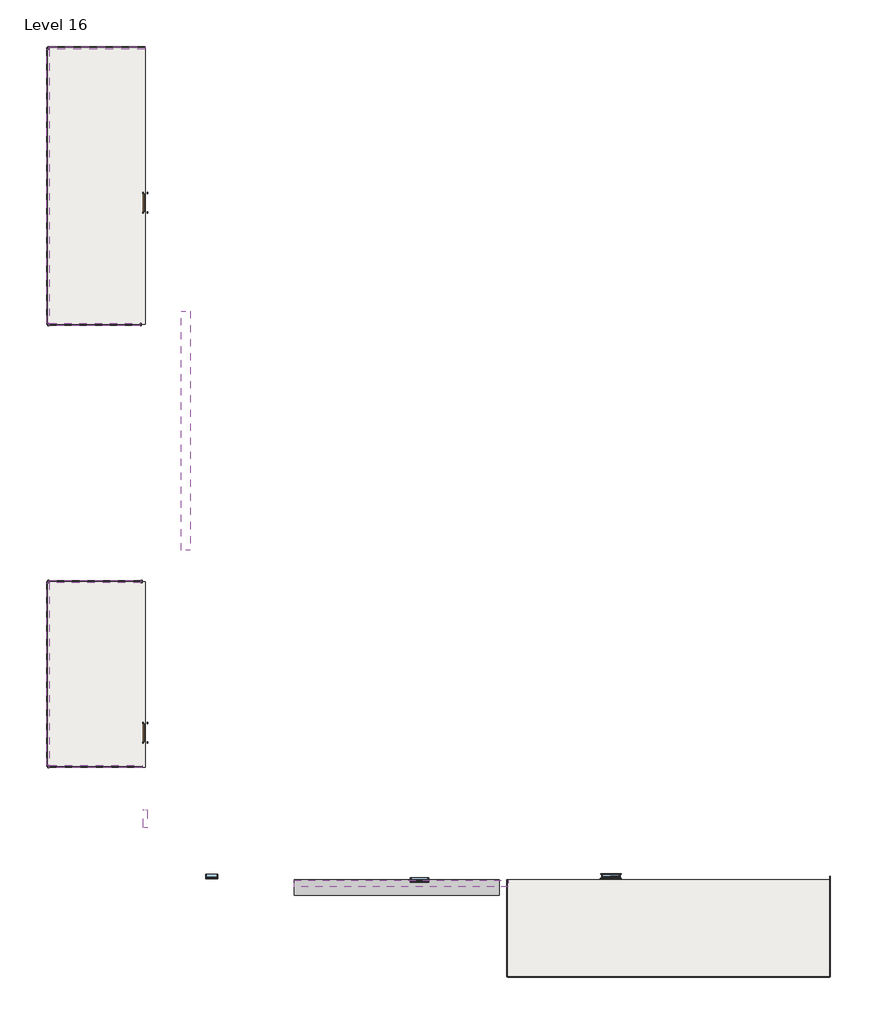
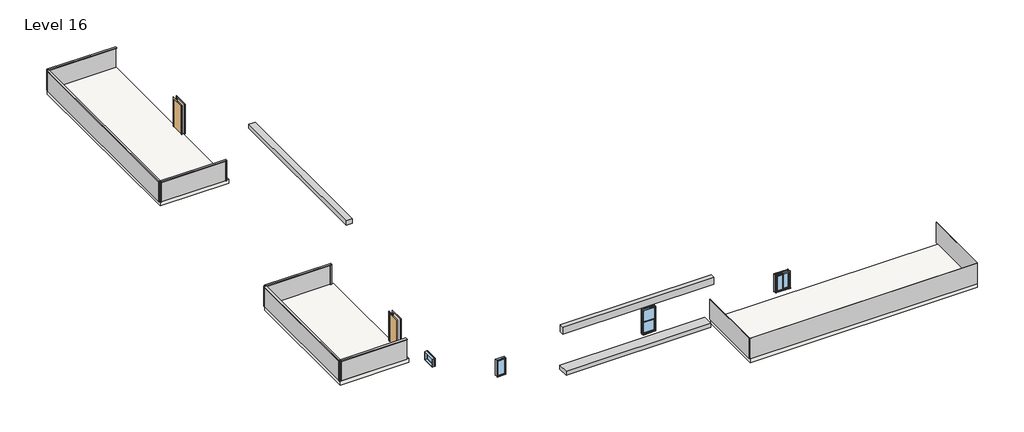
# One storey: 16 members, 9 plates, 4 windows, 3 proxies, 3 slabs, 2 doors.
"""IFC4 building model written with IfcOpenShell, lengths in millimetres."""

from ifc_helpers import new_model, si_unit, frame, origin, place, context, project, spatial, polyline, outline, extrude, transform, mapped, element, save
from components import generic_models_14_generic_models_14_5b98b352, generic_models_3_generic_models_3_29ab51b9, generic_models_4_generic_models_4_efb5897f, door_54dd4da4, member_a0ba9e48, member_4491d118, member_315671ef, member_50e41c3e, member_44cf4dfe, member_4960e788, member_0f997902, system_panel_glazed_29cdcffd, system_panel_glazed_0e082344, system_panel_glazed_4760f0d8, system_panel_glazed_82bc3a22, system_panel_glazed_a411ffd8, system_panel_glazed_3a6cb6e4, system_panel_glazed_7f285cc4, system_panel_glazed_1f6fd899, system_panel_glazed_96c75d75, window_f274a882, window_57c3ee1c, window_78885257, window_54100e87

model = new_model("IFC4")

# Units and contexts
model_context = context("Model", 3, world=origin())
ifc_project = project(units=[si_unit("LENGTHUNIT", "METRE", prefix="MILLI")], contexts=[model_context])

# Site, building, storey
site = spatial("IfcSite", under=ifc_project)
building = spatial("IfcBuilding", under=site)
storey = spatial("IfcBuildingStorey", under=building, Name="Level 16", Elevation=26517.6)

# Proxies
placement = place(None, origin())
generic_models_14_generic_models_14_shape = generic_models_14_generic_models_14_5b98b352(model_context)
element("IfcBuildingElementProxy", 1, Name="Generic Models 14 : Generic Models 14", ObjectType="Generic Models 14 : Generic Models 14", at=placement, inside=storey, context=model_context, shape_type="MappedRepresentation", body=[
    mapped(generic_models_14_generic_models_14_shape, transform((0.0, 0.0, 0.0), x_axis=(1.0, 0.0, 0.0), y_axis=(0.0, 1.0, 0.0), z_axis=(0.0, 0.0, 1.0))),
])
generic_models_3_generic_models_3_shape = generic_models_3_generic_models_3_29ab51b9(model_context)
element("IfcBuildingElementProxy", 2, Name="Generic Models 3 : Generic Models 3", ObjectType="Generic Models 3 : Generic Models 3", at=placement, inside=storey, context=model_context, shape_type="MappedRepresentation", body=[
    mapped(generic_models_3_generic_models_3_shape, transform((0.0, 0.0, 0.0), x_axis=(1.0, 0.0, 0.0), y_axis=(0.0, 1.0, 0.0), z_axis=(0.0, 0.0, 1.0))),
])
generic_models_4_generic_models_4_shape = generic_models_4_generic_models_4_efb5897f(model_context)
element("IfcBuildingElementProxy", 3, Name="Generic Models 4 : Generic Models 4", ObjectType="Generic Models 4 : Generic Models 4", at=placement, inside=storey, context=model_context, shape_type="MappedRepresentation", body=[
    mapped(generic_models_4_generic_models_4_shape, transform((0.0, 0.0, 0.0), x_axis=(1.0, 0.0, 0.0), y_axis=(0.0, 1.0, 0.0), z_axis=(0.0, 0.0, 1.0))),
])

# Doors
door_shape = door_54dd4da4(model_context)
element("IfcDoor", 4, ObjectType="Single-Flush : 36\" x 84\"", at=placement, inside=storey, context=model_context, shape_type="MappedRepresentation", body=[
    mapped(door_shape, transform((-15175.038074, 13037.8014639, 26517.6), x_axis=(0.0, 1.0, 0.0), y_axis=(-1.0, 0.0, 0.0), z_axis=(0.0, 0.0, 1.0))),
])
element("IfcDoor", 5, ObjectType="Single-Flush : 36\" x 84\"", at=placement, inside=storey, context=model_context, shape_type="MappedRepresentation", body=[
    mapped(door_shape, transform((-15175.038074, -13547.7915889, 26517.6), x_axis=(0.0, 1.0, 0.0), y_axis=(-1.0, 0.0, 0.0), z_axis=(0.0, 0.0, 1.0))),
])

# Members
member_shape = member_a0ba9e48(model_context)
element("IfcMember", 6, ObjectType="Rectangular Mullion : 2.5\" x 5\" rectangular", at=placement, inside=storey, context=model_context, shape_type="MappedRepresentation", body=[
    mapped(member_shape, transform((-15175.038074, 20810.2014639, 28041.6), x_axis=(0.0, 0.0, 1.0), y_axis=(0.0, -1.0, 0.0), z_axis=(1.0, 0.0, 0.0))),
])
member_2_shape = member_4491d118(model_context)
element("IfcMember", 7, ObjectType="Rectangular Mullion : 2.5\" x 5\" rectangular", at=placement, inside=storey, context=model_context, shape_type="MappedRepresentation", body=[
    mapped(member_2_shape, transform((-20051.838074, 20810.2014639, 26517.6), x_axis=(0.0, 1.0, 0.0), y_axis=(1.0, 0.0, 0.0), z_axis=(0.0, 0.0, -1.0))),
])
element("IfcMember", 8, ObjectType="Rectangular Mullion : 2.5\" x 5\" rectangular", at=placement, inside=storey, context=model_context, shape_type="MappedRepresentation", body=[
    mapped(member_2_shape, transform((-20051.838074, 6941.8014639, 26517.6), x_axis=(-1.0, 0.0, 0.0), y_axis=(0.0, 1.0, 0.0), z_axis=(0.0, 0.0, -1.0))),
])
element("IfcMember", 9, ObjectType="Rectangular Mullion : 2.5\" x 5\" rectangular", at=placement, inside=storey, context=model_context, shape_type="MappedRepresentation", body=[
    mapped(member_2_shape, transform((-20051.838074, -5966.8213044, 26517.6), x_axis=(0.0, 1.0, 0.0), y_axis=(1.0, 0.0, 0.0), z_axis=(0.0, 0.0, -1.0))),
])
element("IfcMember", 10, ObjectType="Rectangular Mullion : 2.5\" x 5\" rectangular", at=placement, inside=storey, context=model_context, shape_type="MappedRepresentation", body=[
    mapped(member_2_shape, transform((-15327.438074, -5966.8213044, 26517.6), x_axis=(1.0, 0.0, 0.0), y_axis=(0.0, -1.0, 0.0), z_axis=(0.0, 0.0, -1.0))),
])
element("IfcMember", 11, ObjectType="Rectangular Mullion : 2.5\" x 5\" rectangular", at=placement, inside=storey, context=model_context, shape_type="MappedRepresentation", body=[
    mapped(member_2_shape, transform((-20051.838074, -15231.4713044, 26517.6), x_axis=(-1.0, 0.0, 0.0), y_axis=(0.0, 1.0, 0.0), z_axis=(0.0, 0.0, -1.0))),
])
element("IfcMember", 12, ObjectType="Rectangular Mullion : 2.5\" x 5\" rectangular", at=placement, inside=storey, context=model_context, shape_type="MappedRepresentation", body=[
    mapped(member_2_shape, transform((-20051.838074, 20810.2014639, 28041.6), x_axis=(-1.0, 0.0, 0.0), y_axis=(0.0, -1.0, 0.0), z_axis=(0.0, 0.0, 1.0))),
])
element("IfcMember", 13, ObjectType="Rectangular Mullion : 2.5\" x 5\" rectangular", at=placement, inside=storey, context=model_context, shape_type="MappedRepresentation", body=[
    mapped(member_2_shape, transform((-20051.838074, 6941.8014639, 28041.6), x_axis=(0.0, -1.0, 0.0), y_axis=(1.0, 0.0, 0.0), z_axis=(0.0, 0.0, 1.0))),
])
element("IfcMember", 14, ObjectType="Rectangular Mullion : 2.5\" x 5\" rectangular", at=placement, inside=storey, context=model_context, shape_type="MappedRepresentation", body=[
    mapped(member_2_shape, transform((-15360.4013228, 6941.8014639, 28041.6), x_axis=(1.0, 0.0, 0.0), y_axis=(0.0, 1.0, 0.0), z_axis=(0.0, 0.0, 1.0))),
])
element("IfcMember", 15, ObjectType="Rectangular Mullion : 2.5\" x 5\" rectangular", at=placement, inside=storey, context=model_context, shape_type="MappedRepresentation", body=[
    mapped(member_2_shape, transform((-20051.838074, -5966.8213044, 28041.6), x_axis=(-1.0, 0.0, 0.0), y_axis=(0.0, -1.0, 0.0), z_axis=(0.0, 0.0, 1.0))),
])
element("IfcMember", 16, ObjectType="Rectangular Mullion : 2.5\" x 5\" rectangular", at=placement, inside=storey, context=model_context, shape_type="MappedRepresentation", body=[
    mapped(member_2_shape, transform((-20051.838074, -15231.4713044, 28041.6), x_axis=(0.0, -1.0, 0.0), y_axis=(1.0, 0.0, 0.0), z_axis=(0.0, 0.0, 1.0))),
])
member_3_shape = member_315671ef(model_context)
element("IfcMember", 17, ObjectType="Rectangular Mullion : 2.5\" x 5\" rectangular", at=placement, inside=storey, context=model_context, shape_type="MappedRepresentation", body=[
    mapped(member_3_shape, transform((-20051.838074, 20746.7014639, 28041.6), x_axis=(0.0, 0.0, 1.0), y_axis=(1.0, 0.0, 0.0), z_axis=(0.0, 1.0, 0.0))),
])
member_4_shape = member_50e41c3e(model_context)
element("IfcMember", 18, ObjectType="Rectangular Mullion : 2.5\" x 5\" rectangular", at=placement, inside=storey, context=model_context, shape_type="MappedRepresentation", body=[
    mapped(member_4_shape, transform((-19988.338074, 6941.8014639, 28041.6), x_axis=(0.0, 0.0, 1.0), y_axis=(0.0, 1.0, 0.0), z_axis=(-1.0, 0.0, 0.0))),
])
member_5_shape = member_44cf4dfe(model_context)
element("IfcMember", 19, ObjectType="Rectangular Mullion : 2.5\" x 5\" rectangular", at=placement, inside=storey, context=model_context, shape_type="MappedRepresentation", body=[
    mapped(member_5_shape, transform((-15390.938074, -5966.8213044, 28041.6), x_axis=(0.0, 0.0, 1.0), y_axis=(0.0, -1.0, 0.0), z_axis=(1.0, 0.0, 0.0))),
])
member_6_shape = member_4960e788(model_context)
element("IfcMember", 20, ObjectType="Rectangular Mullion : 2.5\" x 5\" rectangular", at=placement, inside=storey, context=model_context, shape_type="MappedRepresentation", body=[
    mapped(member_6_shape, transform((-20051.838074, -6030.3213044, 28041.6), x_axis=(0.0, 0.0, 1.0), y_axis=(1.0, 0.0, 0.0), z_axis=(0.0, 1.0, 0.0))),
])
member_7_shape = member_0f997902(model_context)
element("IfcMember", 21, ObjectType="Rectangular Mullion : 2.5\" x 5\" rectangular", at=placement, inside=storey, context=model_context, shape_type="MappedRepresentation", body=[
    mapped(member_7_shape, transform((-19988.338074, -15231.4713044, 28041.6), x_axis=(0.0, 0.0, 1.0), y_axis=(0.0, 1.0, 0.0), z_axis=(-1.0, 0.0, 0.0))),
])

# Plates
system_panel_glazed_shape = system_panel_glazed_29cdcffd(model_context)
element("IfcPlate", 22, ObjectType="System Panel : Glazed", at=placement, inside=storey, context=model_context, shape_type="MappedRepresentation", body=[
    mapped(system_panel_glazed_shape, transform((19140.361926, -23258.7985361, 26517.6), x_axis=(0.0, -1.0, 0.0), y_axis=(1.0, 0.0, 0.0), z_axis=(0.0, 0.0, 1.0))),
])
system_panel_glazed_2_shape = system_panel_glazed_0e082344(model_context)
element("IfcPlate", 23, ObjectType="System Panel : Glazed", at=placement, inside=storey, context=model_context, shape_type="MappedRepresentation", body=[
    mapped(system_panel_glazed_2_shape, transform((11075.861926, -25773.3985361, 26517.6), x_axis=(-1.0, 0.0, 0.0), y_axis=(0.0, -1.0, 0.0), z_axis=(0.0, 0.0, 1.0))),
])
system_panel_glazed_3_shape = system_panel_glazed_4760f0d8(model_context)
element("IfcPlate", 24, ObjectType="System Panel : Glazed", at=placement, inside=storey, context=model_context, shape_type="MappedRepresentation", body=[
    mapped(system_panel_glazed_3_shape, transform((3011.361926, -23347.6985361, 26517.6), x_axis=(0.0, 1.0, 0.0), y_axis=(-1.0, 0.0, 0.0), z_axis=(0.0, 0.0, 1.0))),
])
system_panel_glazed_4_shape = system_panel_glazed_82bc3a22(model_context)
element("IfcPlate", 25, ObjectType="System Panel : Glazed", at=placement, inside=storey, context=model_context, shape_type="MappedRepresentation", body=[
    mapped(system_panel_glazed_4_shape, transform((-17581.688074, 20810.2014639, 26517.6), x_axis=(1.0, 0.0, 0.0), y_axis=(0.0, 1.0, 0.0), z_axis=(0.0, 0.0, 1.0))),
])
system_panel_glazed_5_shape = system_panel_glazed_a411ffd8(model_context)
element("IfcPlate", 26, ObjectType="System Panel : Glazed", at=placement, inside=storey, context=model_context, shape_type="MappedRepresentation", body=[
    mapped(system_panel_glazed_5_shape, transform((-20051.838074, 13876.0014639, 26517.6), x_axis=(0.0, 1.0, 0.0), y_axis=(-1.0, 0.0, 0.0), z_axis=(0.0, 0.0, 1.0))),
])
system_panel_glazed_6_shape = system_panel_glazed_3a6cb6e4(model_context)
element("IfcPlate", 27, ObjectType="System Panel : Glazed", at=placement, inside=storey, context=model_context, shape_type="MappedRepresentation", body=[
    mapped(system_panel_glazed_6_shape, transform((-17706.1196984, 6941.8014639, 26517.6), x_axis=(-1.0, 0.0, 0.0), y_axis=(0.0, -1.0, 0.0), z_axis=(0.0, 0.0, 1.0))),
])
system_panel_glazed_7_shape = system_panel_glazed_7f285cc4(model_context)
element("IfcPlate", 28, ObjectType="System Panel : Glazed", at=placement, inside=storey, context=model_context, shape_type="MappedRepresentation", body=[
    mapped(system_panel_glazed_7_shape, transform((-17689.638074, -5966.8213044, 26517.6), x_axis=(1.0, 0.0, 0.0), y_axis=(0.0, 1.0, 0.0), z_axis=(0.0, 0.0, 1.0))),
])
system_panel_glazed_8_shape = system_panel_glazed_1f6fd899(model_context)
element("IfcPlate", 29, ObjectType="System Panel : Glazed", at=placement, inside=storey, context=model_context, shape_type="MappedRepresentation", body=[
    mapped(system_panel_glazed_8_shape, transform((-20051.838074, -10599.1463044, 26517.6), x_axis=(0.0, 1.0, 0.0), y_axis=(-1.0, 0.0, 0.0), z_axis=(0.0, 0.0, 1.0))),
])
system_panel_glazed_9_shape = system_panel_glazed_96c75d75(model_context)
element("IfcPlate", 30, ObjectType="System Panel : Glazed", at=placement, inside=storey, context=model_context, shape_type="MappedRepresentation", body=[
    mapped(system_panel_glazed_9_shape, transform((-17657.888074, -15231.4713044, 26517.6), x_axis=(-1.0, 0.0, 0.0), y_axis=(0.0, -1.0, 0.0), z_axis=(0.0, 0.0, 1.0))),
])

# Slabs
element("IfcSlab", 31, ObjectType="Generic - 12\"", at=placement, inside=storey, context=model_context, shape_type="SweptSolid", body=[
    extrude(outline(polyline([(3011.361926, -20921.9985361), (19165.761926, -20921.9985361), (19165.761926, -25798.7985361), (3011.361926, -25798.7985361), (3011.361926, -20921.9985361)])), frame((0.0, 0.0, 26212.8), z_axis=(0.0, 0.0, 1.0), x_axis=(1.0, 0.0, 0.0)), (0.0, 0.0, 1.0), 304.8),
])
element("IfcSlab", 32, ObjectType="Generic - 12\"", at=placement, inside=storey, context=model_context, shape_type="SweptSolid", body=[
    extrude(outline(polyline([(-20051.838074, -15263.2213044), (-20051.838074, -5966.8213044), (-15175.038074, -5966.8213044), (-15175.038074, -15263.2213044), (-20051.838074, -15263.2213044)])), frame((0.0, 0.0, 26212.8), z_axis=(0.0, 0.0, 1.0), x_axis=(1.0, 0.0, 0.0)), (0.0, 0.0, 1.0), 304.8),
])
element("IfcSlab", 33, ObjectType="Generic - 12\"", at=placement, inside=storey, context=model_context, shape_type="SweptSolid", body=[
    extrude(outline(polyline([(-20051.838074, 20810.2014639), (-15175.038074, 20810.2014639), (-15175.038074, 6941.8014639), (-20051.838074, 6941.8014639), (-20051.838074, 20810.2014639)])), frame((0.0, 0.0, 26212.8), z_axis=(0.0, 0.0, 1.0), x_axis=(1.0, 0.0, 0.0)), (0.0, 0.0, 1.0), 304.8),
])

# Windows
window_shape = window_f274a882(model_context)
element("IfcWindow", 34, ObjectType="Double Hung : 36\" x 72\"", at=placement, inside=storey, context=model_context, shape_type="MappedRepresentation", body=[
    mapped(window_shape, transform((-1408.238074, -20921.9985361, 26806.9086033), x_axis=(-1.0, 0.0, 0.0), y_axis=(0.0, -1.0, 0.0), z_axis=(0.0, 0.0, 1.0))),
])
window_2_shape = window_57c3ee1c(model_context)
element("IfcWindow", 35, ObjectType="Fixed : 36\" x 24\"", at=placement, inside=storey, context=model_context, shape_type="MappedRepresentation", body=[
    mapped(window_2_shape, transform((-15175.038074, -17892.1213044, 26824.6132762), x_axis=(0.0, -1.0, 0.0), y_axis=(1.0, 0.0, 0.0), z_axis=(0.0, 0.0, 1.0))),
])
window_3_shape = window_78885257(model_context)
element("IfcWindow", 36, ObjectType="Instance - Fixed : 24\" x 48\"", at=placement, inside=storey, context=model_context, shape_type="MappedRepresentation", body=[
    mapped(window_3_shape, transform((-11860.338074, -20744.1985361, 26517.6), x_axis=(-1.0, 0.0, 0.0), y_axis=(0.0, -1.0, 0.0), z_axis=(0.0, 0.0, 1.0))),
])
window_4_shape = window_54100e87(model_context)
element("IfcWindow", 37, ObjectType="Slider with Trim : 36\" x 48\"", at=placement, inside=storey, context=model_context, shape_type="MappedRepresentation", body=[
    mapped(window_4_shape, transform((8192.961926, -20744.1985361, 25925.0536631), x_axis=(-1.0, 0.0, 0.0), y_axis=(0.0, -1.0, 0.0), z_axis=(0.0, 0.0, 1.0))),
])

save(model, "model.ifc")

# Revit data of these elements
# Type "Single-Flush : 36\" x 84\""
#   Type Mark = "1"
#   Construction Type Id = "MDOOR"
#   Assembly Code = "C1020"
#   Analytic Construction = "Metal"
#   Thickness = 0' - 2"
#   Heat Transfer Coefficient (U) = 0.651978 BTU/(h·ft²·°F)
#   Height = 7' - 0"
#   Trim Projection Ext = 0' - 1"
#   Trim Projection Int = 0' - 1"
#   Trim Width = 0' - 3"
#   Width = 3' - 0"
#   Define Thermal Properties by = 1
#   Door Material = Door - Panel
#   Frame Material = Door - Frame
#   Visual Light Transmittance = 0
#   Solar Heat Gain Coefficient = 0
#   Function = (empty or 0)
#   Wall Closure = (empty or 0)
# Type "Rectangular Mullion : 2.5\" x 5\" rectangular"
#   built-in parameter 1007304 = 0.416667 (stored number, unit not read)
#   built-in parameter 1007301 = 0.104167 (stored number, unit not read)
#   built-in parameter 1007300 = 0.104167 (stored number, unit not read)
# Type "System Panel : Glazed"
#   Construction Type Id = "GSP4R"
#   Analytic Construction = "1/8 in Pilkington single glazing"
#   Visual Light Transmittance = 0.9
#   Solar Heat Gain Coefficient = 0.86
#   Heat Transfer Coefficient (U) = 1.18115 BTU/(h·ft²·°F)
# Type "Generic - 12\""
#   Assembly Code = "B1010"
#   Function = 0
#   Layers, outside or top first: 1' - 0" no material (function 1)
# Type "Double Hung : 36\" x 72\""
#   Type Mark = "18"
#   Construction Type Id = "GSP4R"
#   Assembly Code = "B2020100"
#   Analytic Construction = "1/8 in Pilkington single glazing"
#   Visual Light Transmittance = 0.9
#   Solar Heat Gain Coefficient = 0.78
#   Heat Transfer Coefficient (U) = 0.6496 BTU/(h·ft²·°F)
#   Height = 6' - 0"
#   Default Sill Height = 1' - 0"
#   Width = 3' - 0"
#   Window Inset = 0' - 0 3/4"
#   Define Thermal Properties by = 1
#   Glass Pane Material = Glass
#   Sash Material = Sash
#   Description = (empty or 0)
#   Wall Closure = (empty or 0)
# Type "Fixed : 36\" x 24\""
#   Type Mark = "8"
#   Construction Type Id = "GSP4R"
#   Assembly Code = "B2020100"
#   Analytic Construction = "1/8 in Pilkington single glazing"
#   Visual Light Transmittance = 0.9
#   Solar Heat Gain Coefficient = 0.78
#   Heat Transfer Coefficient (U) = 0.6496 BTU/(h·ft²·°F)
#   Height = 2' - 0"
#   Default Sill Height = 3' - 0"
#   Width = 3' - 0"
#   Window Inset = 0' - 0 3/4"
#   Define Thermal Properties by = 1
#   Glass Pane Material = Glass
#   Sash Material = Sash
#   Wall Closure = (empty or 0)
# Type "Instance - Fixed : 24\" x 48\""
#   Type Mark = "19"
#   Construction Type Id = "GSP4R"
#   Assembly Code = "B2020100"
#   Analytic Construction = "1/8 in Pilkington single glazing"
#   Visual Light Transmittance = 0.9
#   Thermal Resistance (R) = 0.8466 (h·ft²·°F)/BTU
#   Solar Heat Gain Coefficient = 0.86
#   Heat Transfer Coefficient (U) = 1.1812 BTU/(h·ft²·°F)
#   Height [instance default] = 4' - 0"
#   Default Sill Height = 3' - 0"
#   Width [instance default] = 2' - 0"
#   Window Inset = 0' - 0 3/4"
#   Define Thermal Properties by = 1
#   Glass Pane Material = Glass
#   Sash Material = Sash
#   Wall Closure = (empty or 0)
# Type "Slider with Trim : 36\" x 48\""
#   Type Mark = "22"
#   Construction Type Id = "GSP4R"
#   Assembly Code = "B2020100"
#   Analytic Construction = "1/8 in Pilkington single glazing"
#   Visual Light Transmittance = 0.9
#   Solar Heat Gain Coefficient = 0.78
#   Heat Transfer Coefficient (U) = 0.6496 BTU/(h·ft²·°F)
#   Height = 4' - 0"
#   Default Sill Height = 3' - 0"
#   Trim Projection - Ext. = 0' - 0 3/4"
#   Trim Projection - Int. = 0' - 0 3/4"
#   Trim Width - Exterior = 0' - 3 1/2"
#   Trim Width - Interior = 0' - 3 1/2"
#   Width = 3' - 0"
#   Window Inset = 0' - 0 3/4"
#   Define Thermal Properties by = 1
#   Glass Pane Material = Glass
#   Sash Material = Sash
#   Trim Exterior Material = Trim
#   Trim Interior Material = Trim
#   Wall Closure = (empty or 0)
# Element 1 (IfcBuildingElementProxy, "Generic Models 14 : Generic Models 14")
#   Phase Created = New Construction
# Element 2 (IfcBuildingElementProxy, "Generic Models 3 : Generic Models 3")
#   Phase Created = New Construction
# Element 3 (IfcBuildingElementProxy, "Generic Models 4 : Generic Models 4")
#   Phase Created = New Construction
# Elements 4, 5 (IfcDoor, "Single-Flush : 36\" x 84\"")
#   Phase Created = New Construction
#   Materials on its faces: "Door - Frame", "Door - Panel"
# Elements 6, 7, 8, 9, 10, 11, 12, 13, 14, 15, 16, 17, 18, 19, 20, 21 (IfcMember, "Rectangular Mullion : 2.5\" x 5\" rectangular")
#   Phase Created = New Construction
#   Materials on its faces: "Aluminum"
# Elements 22, 23, 24, 25, 26, 27, 28, 29, 30 (IfcPlate, "System Panel : Glazed")
#   Phase Created = New Construction
#   Materials on its faces: "Glass"
# Elements 31, 32, 33 (IfcSlab, "Generic - 12\"")
#   built-in parameter 1001955 = 3.14159 (stored number, unit not read)
#   Height Offset From Level = 0' - 0"
#   Phase Created = New Construction
#   Materials on its faces: "Default Floor"
# Element 34 (IfcWindow, "Double Hung : 36\" x 72\"")
#   Mark = "5"
#   Phase Created = New Construction
#   Materials on its faces: "Sash", "Glass"
# Element 35 (IfcWindow, "Fixed : 36\" x 24\"")
#   Mark = "70"
#   Phase Created = New Construction
#   Materials on its faces: "Sash", "Glass"
# Element 36 (IfcWindow, "Instance - Fixed : 24\" x 48\"")
#   Mark = "15"
#   Width = 2' - 0"
#   Height = 4' - 0"
#   Phase Created = New Construction
#   Materials on its faces: "Sash", "Glass"
# Element 37 (IfcWindow, "Slider with Trim : 36\" x 48\"")
#   Mark = "26"
#   Phase Created = New Construction
#   Materials on its faces: "Sash", "Trim", "Glass"
# Materials
#   "Door - Panel": class "Wood", colour RGB 210 159 95, transparency 0
#   "Door - Frame": colour RGB 118 70 51, transparency 0
#   "Glass": class "Glass", colour RGB 0 128 192, transparency 0.75, Description = "Soda Lime Glass", Cost = 0
#   "Sash": class "Wood", colour RGB 224 178 126, transparency 0
#   "Trim": class "Wood", colour RGB 224 178 126, transparency 0
#   "Aluminum": class "Metal", colour RGB 247 247 247, transparency 0, Description = "Aluminum 6061", Cost = 0
#   "Default Floor": colour RGB 128 128 128, transparency 0
